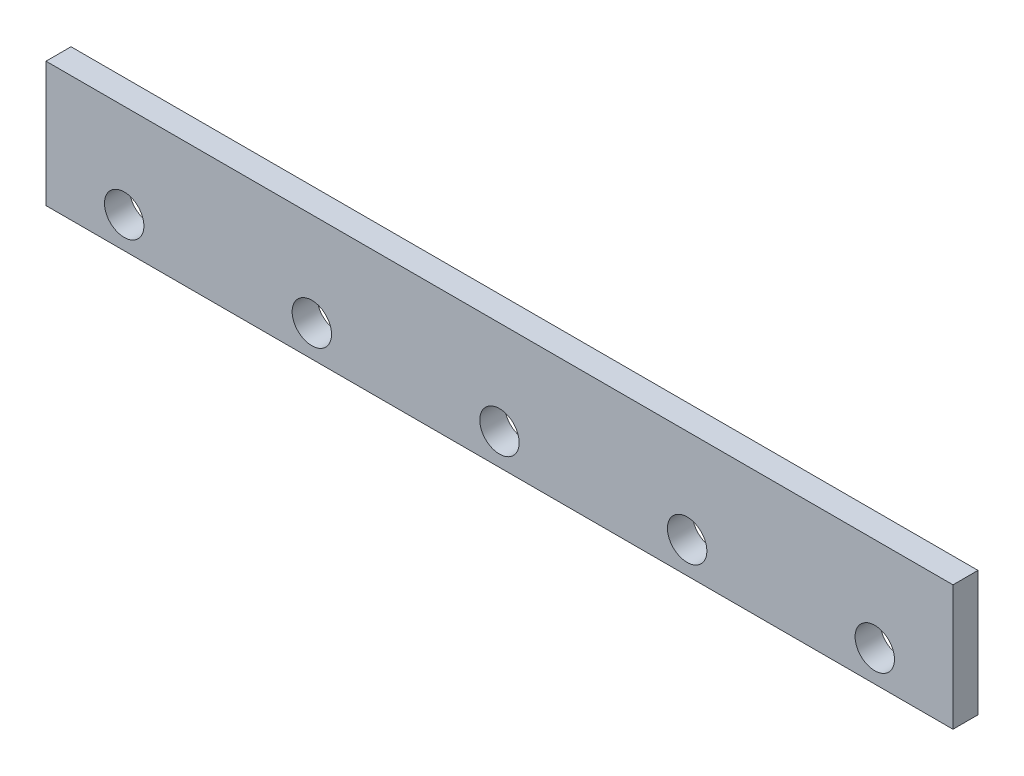
from build123d import *

# Parameters (mm, degrees)
BAR_PROFILE_SKETCH_W             = 580
BAR_PROFILE_SKETCH_H             = 80
FLAT_BAR_580X80X16_DEPTH         = 16
HOLE_ROW_SKETCH_R                = 12.6
THROUGH_HOLES_5X_PITCH_120_DEPTH = 26


with BuildPart() as part:
    # Bar Profile Sketch → Flat Bar 580x80x16 (new body)
    with BuildSketch(Plane.XY):
        Rectangle(BAR_PROFILE_SKETCH_W, BAR_PROFILE_SKETCH_H)
    extrude(amount=FLAT_BAR_580X80X16_DEPTH)

    # Hole Row Sketch → Through Holes 5x Pitch 120 (cut)
    with BuildSketch(Plane.XY.offset(16)):
        with Locations((-240, -20)):
            Circle(HOLE_ROW_SKETCH_R)
        with Locations((-120, -20)):
            Circle(HOLE_ROW_SKETCH_R)
        with Locations((0, -20)):
            Circle(HOLE_ROW_SKETCH_R)
        with Locations((120, -20)):
            Circle(HOLE_ROW_SKETCH_R)
        with Locations((240, -20)):
            Circle(HOLE_ROW_SKETCH_R)
    extrude(amount=-THROUGH_HOLES_5X_PITCH_120_DEPTH, mode=Mode.SUBTRACT)


solid = part.part
